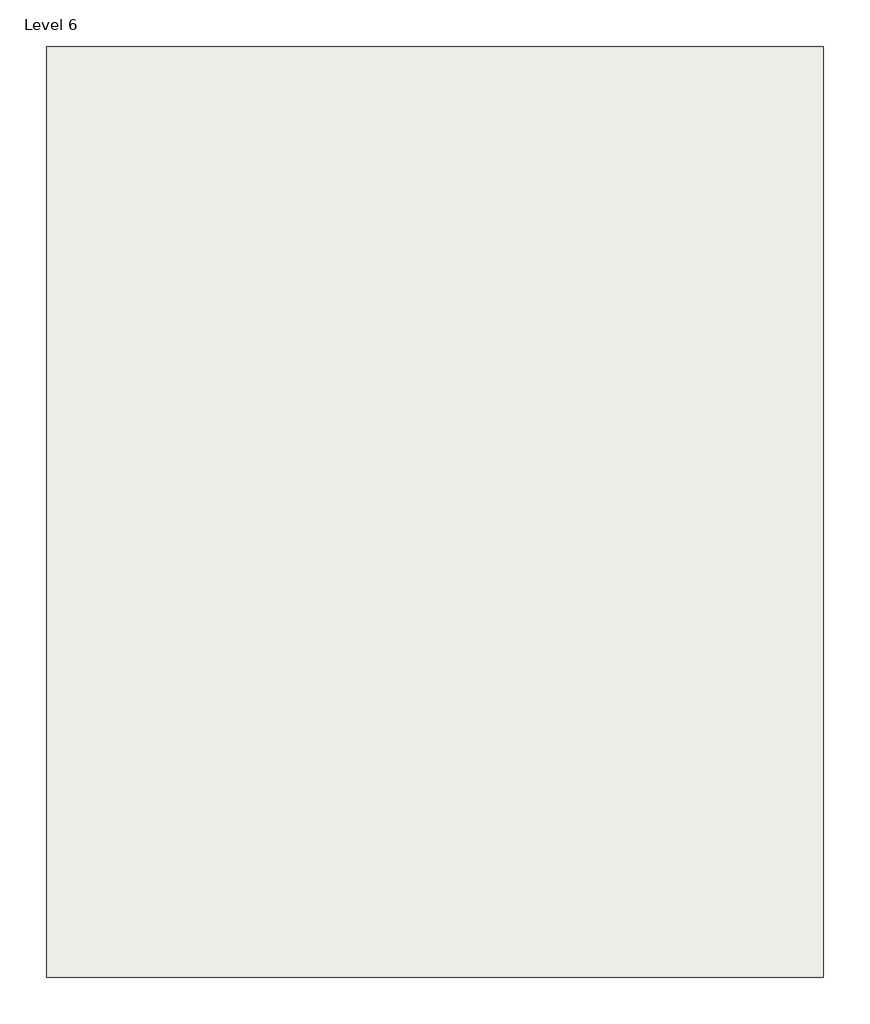
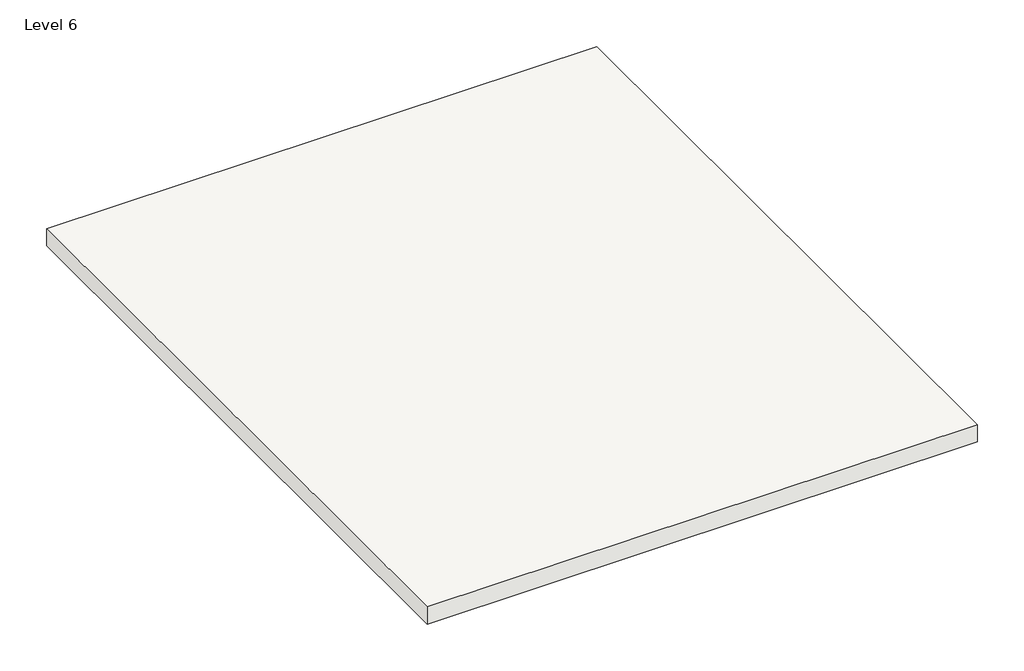
# One storey: 1 roof.
"""IFC4 building model written with IfcOpenShell, lengths in millimetres."""

from ifc_helpers import new_model, si_unit, frame, origin, place, context, project, spatial, polyline, outline, extrude, element, save

model = new_model("IFC4")

# Units and contexts
model_context = context("Model", 3, world=origin())
ifc_project = project(units=[si_unit("LENGTHUNIT", "METRE", prefix="MILLI")], contexts=[model_context])

# Site, building, storey
site = spatial("IfcSite", under=ifc_project)
building = spatial("IfcBuilding", under=site)
storey = spatial("IfcBuildingStorey", under=building, Name="Level 6", Elevation=6248.4)

# Roof
placement = place(None, origin())
element("IfcRoof", 1, ObjectType="6\"", at=placement, inside=storey, context=model_context, shape_type="SweptSolid", body=[
    extrude(outline(polyline([(-4629.1116656, 12667.0455153), (-6.3116656, 12667.0455153), (-6.3116656, 7129.8455153), (-4629.1116656, 7129.8455153), (-4629.1116656, 12667.0455153)])), frame((0.0, 0.0, 6248.4), z_axis=(0.0, 0.0, 1.0), x_axis=(1.0, 0.0, 0.0)), (0.0, 0.0, 1.0), 152.4),
])

save(model, "model.ifc")

# Revit data of these elements
# Type "6\""
#   Assembly Code = "B1020"
#   Layers, outside or top first: 0' - 6" no material (function 1)
# Element 1 (IfcRoof, "6\"")
#   built-in parameter 1001705 = 21 (stored number, unit not read)
#   built-in parameter 1001710 = 33615
#   Phase Created = New Construction
#   Materials on its faces: "Default Roof"
# Materials
#   "Default Roof": colour RGB 88 101 114, transparency 0, Cost = 0
